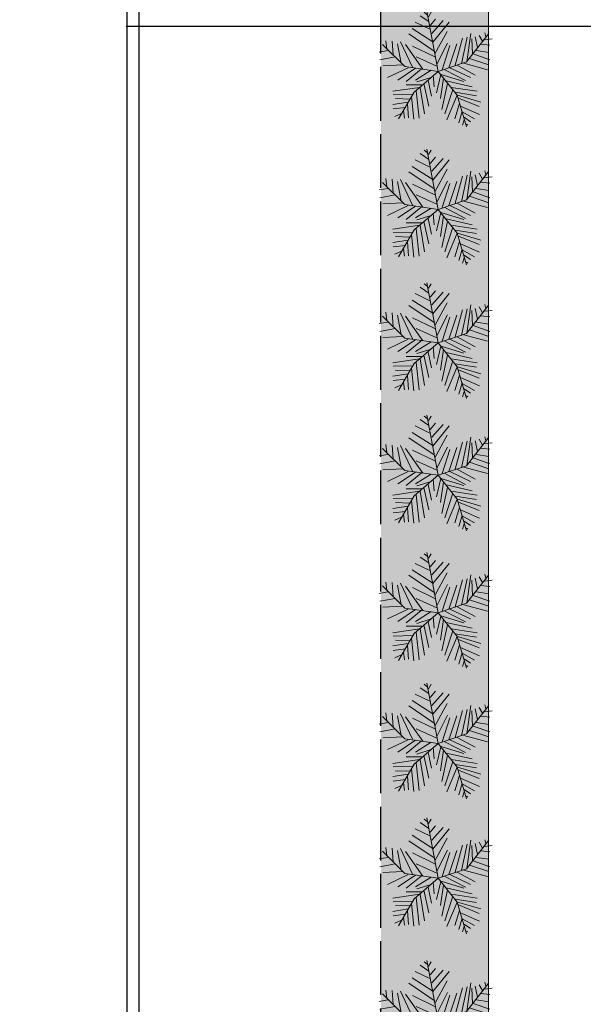
# Model space of a CAD drawing. Units: inches. Extents: x 853 to 1550, y 485 to 1596.
# Tile 12 of 18: x 853 to 979, y 1208 to 1428. Entities that reach past the tile are written whole.
import ezdxf

# ---------------------------------------------------------------- set-up
doc = ezdxf.new("R2010")
doc.units = ezdxf.units.IN
doc.header["$MEASUREMENT"] = 0
doc.linetypes.add('ACAD_ISO02W100', pattern=[15, 12, -3])
for name, color, linetype, lineweight in [('A-ANNO-DIMS', 2, 'Continuous', 18), ('C-PROP', 8, 'ACAD_ISO02W100', 25), ('L-PLNT-TREE', 106, 'Continuous', 13), ('lawn', 106, 'Continuous', 18)]:
    doc.layers.add(name, color=color, linetype=linetype, lineweight=lineweight)
doc.layers.add('L-PLNT-PATT', color=85, linetype='Continuous', lineweight=13, true_color=0x58ba48)
doc.styles.get("Standard").update_dxf_attribs({"font": 'arial.ttf'})
doc.dimstyles.get("Standard").update_dxf_attribs({"dimtxt": 8, "dimasz": 0.18, "dimexe": 0.18, "dimexo": 0.0625, "dimgap": 0.09, "dimtad": 0, "dimtih": 1, "dimtoh": 1, "dimzin": 0, "dimdsep": 46, "dimlunit": 3, "dimtxsty": 'Standard', "dimcen": 0.09, "dimadec": 0, "dimazin": 0, "dimtfac": 1, "dimtofl": 0, "dimtmove": 0, "dimatfit": 3, "dimfxl": 1, "dimtolj": 1, "dimtzin": 0, "dimarcsym": 0})

# ---------------------------------------------------------------- blocks, each defined once
blk = doc.blocks.new('*U18')
for p, q in [((-10.186, 53.64), (-13.084, 55.962)), ((0, 0), (-10.5, 57)), ((-9.099, 51.782), (-6.563, 55.962)), ((-7.288, 39.707), (-21.778, 46.673)), ((-8.737, 47.138), (-17.069, 52.711)), ((-7.65, 43.423), (-2.578, 49.46)), ((-5.839, 35.992), (4.667, 48.067)), ((-5.114, 27.632), (10.463, 46.673)), ((-5.114, 28.097), (-24.676, 40.636)), ((-2.941, 16.486), (8.652, 37.85)), ((-48.585, 21.131), (-49.309, 29.026)), ((-43.513, 28.561), (-42.427, 15.558)), ((-35.544, 28.097), (-24.314, 3.947)), ((-3.665, 19.273), (-27.574, 35.527)), ((16.259, 5.805), (23.142, 31.348)), ((22.055, 7.198), (27.489, 32.277)), ((27, 9), (48, 36)), ((27.127, 9.056), (31.112, 35.992)), ((31.836, 30.883), (32.561, 16.486)), ((35.096, 32.741), (37.27, 22.524)), ((38.719, 34.134), (41.979, 28.561)), ((43.791, 29.954), (51.036, 30.883)), ((44.153, 36.456), (45.239, 32.741)), ((-47.498, 19.737), (-55.83, 18.344)), ((-31.5, 4.5), (-52.5, 25.5)), ((-38.442, 26.239), (-34.819, 7.663)), ((-14.533, 2.09), (-30.834, 25.31)), ((-24.314, 23.917), (-2.941, 13.7)), ((-1.129, 6.734), (9.014, 26.704)), ((3.942, 1.625), (11.187, 24.381)), ((10.101, 3.483), (17.708, 26.239)), ((36.183, 19.737), (48.137, 17.88)), ((40.53, 25.775), (48.862, 24.846)), ((-40.615, 13.7), (-55.105, 10.913)), ((-20.691, 13.7), (-1.129, 4.876)), ((29.662, 12.307), (48.137, 6.269)), ((33.285, 16.486), (48.862, 10.913)), ((-33.37, 6.269), (-52.207, 5.34)), ((-28.299, 3.483), (-47.86, -5.805)), ((-21.416, 3.018), (-38.079, -8.128)), ((0, 0), (-31.5, 4.5)), ((-15.982, 2.09), (-30.11, -9.521)), ((0, 0), (-22.5, -19.5)), ((-6.563, 1.161), (-21.416, -8.128)), ((0, 0), (27, 9)), ((0, 0), (18, -22.5)), ((6.478, 1.625), (26.04, -8.592)), ((11.187, 3.483), (30.749, -5.805)), ((18.07, 5.805), (35.096, -3.483)), ((24.229, 7.663), (46.688, 1.625)), ((-6.563, -5.805), (-19.967, -9.985)), ((-9.461, -8.592), (-6.201, -23.453)), ((-4.752, -3.483), (-3.665, -14.629)), ((2.493, -3.019), (-1.491, -20.202)), ((1.769, -2.555), (24.229, -9.521)), ((5.029, -6.27), (2.131, -25.775)), ((7.565, -9.056), (32.198, -14.629)), ((-17.431, -15.094), (-42.789, -18.809)), ((-15.257, -12.772), (-30.11, -12.772)), ((-20.691, -18.345), (-17.793, -44.352)), ((-17.069, -15.094), (-12.721, -40.172)), ((-13.446, -11.378), (-8.737, -32.741)), ((9.014, -11.378), (3.58, -35.992)), ((14.085, -16.951), (6.478, -40.172)), ((12.274, -15.094), (36.907, -18.809)), ((-24.314, -21.596), (-42.427, -22.06)), ((-26.849, -26.24), (-40.253, -25.775)), ((-22.5, -19.5), (-37.5, -45)), ((-25.038, -23.918), (-22.865, -45.281)), ((18.07, -22.524), (8.289, -45.745)), ((16.259, -19.738), (36.183, -22.989)), ((18, -22.5), (27, -52.5)), ((18.433, -22.524), (40.53, -29.026)), ((19.157, -25.311), (38.719, -33.206)), ((-28.299, -29.026), (-42.789, -31.348)), ((-30.834, -34.135), (-42.427, -35.528)), ((-32.646, -36.921), (-31.921, -44.352)), ((-29.023, -30.884), (-27.936, -43.887)), ((20.244, -30.419), (15.897, -44.816)), ((21.331, -32.741), (39.081, -40.636)), ((-34.457, -39.708), (-40.978, -42.494)), ((22.78, -37.85), (19.519, -48.532)), ((22.78, -38.314), (34.372, -44.816)), ((24.591, -45.745), (23.142, -50.854)), ((24.591, -43.423), (30.749, -47.603)), ((26.764, -49.925), (28.213, -50.854))]:
    blk.add_line(p, q)
blk = doc.blocks.new('*D23')
at = {"layer": 'A-ANNO-DIMS', "color": 0, "lineweight": -2, "transparency": 16777216}
for p, q in [((879.97, 1474.13), (879.75, 1474.13)), ((879.93, 1473.95), (879.93, 1049.11)), ((879.93, 615.92), (879.93, 1040.76)), ((879.97, 615.74), (879.75, 615.74))]:
    blk.add_line(p, q, dxfattribs=at)
at = {"layer": 'A-ANNO-DIMS', "color": 0, "transparency": 16777216}
for points in [[(879.9, 1473.95), (879.96, 1473.95), (879.93, 1474.13)], [(879.9, 615.92), (879.96, 615.92), (879.93, 615.74)]]:
    blk.add_solid(points, dxfattribs=at)
at = {"layer": 'Defpoints', "color": 0, "transparency": 16777216}
for p in [(880.03, 1474.13), (879.93, 615.74), (880.03, 615.74)]:
    blk.add_point(p, dxfattribs=at)
at = {"layer": 'A-ANNO-DIMS', "color": 0, "transparency": 16777216, "insert": (879.93, 1044.94), "char_height": 8, "attachment_point": 5}
blk.add_mtext("\\A1;60'", dxfattribs=at)
blk = doc.blocks.new('*D70')
at = {"layer": 'A-ANNO-DIMS', "color": 0, "lineweight": -2, "transparency": 16777216}
for p, q in [((981.87, 1426.13), (877.09, 1426.13)), ((877.27, 1425.95), (877.27, 1067.22)), ((877.27, 700.05), (877.27, 1058.77)), ((1110.88, 699.87), (877.09, 699.87))]:
    blk.add_line(p, q, dxfattribs=at)
at = {"layer": 'A-ANNO-DIMS', "color": 0, "transparency": 16777216}
for points in [[(877.24, 1425.95), (877.3, 1425.95), (877.27, 1426.13)], [(877.24, 700.05), (877.3, 700.05), (877.27, 699.87)]]:
    blk.add_solid(points, dxfattribs=at)
at = {"layer": 'Defpoints', "color": 0, "transparency": 16777216}
for p in [(981.94, 1426.13), (877.27, 699.87), (1110.94, 699.87)]:
    blk.add_point(p, dxfattribs=at)
at = {"layer": 'A-ANNO-DIMS', "color": 0, "transparency": 16777216, "insert": (877.27, 1063), "char_height": 8, "attachment_point": 5}
blk.add_mtext('\\A1;60\'-6 1/2"', dxfattribs=at)
blk = doc.blocks.new('*D71')
at = {"layer": 'A-ANNO-DIMS', "color": 0, "lineweight": -2, "transparency": 16777216}
for p, q in [((933.87, 1474.13), (877.09, 1474.13)), ((877.27, 1473.95), (877.27, 1015.66)), ((877.27, 549.16), (877.27, 1007.45)), ((933.87, 548.98), (877.09, 548.98))]:
    blk.add_line(p, q, dxfattribs=at)
at = {"layer": 'A-ANNO-DIMS', "color": 0, "transparency": 16777216}
for points in [[(877.24, 1473.95), (877.3, 1473.95), (877.27, 1474.13)], [(877.24, 549.16), (877.3, 549.16), (877.27, 548.98)]]:
    blk.add_solid(points, dxfattribs=at)
at = {"layer": 'Defpoints', "color": 0, "transparency": 16777216}
for p in [(877.27, 1474.13), (933.94, 1474.13), (933.94, 548.98)]:
    blk.add_point(p, dxfattribs=at)
at = {"layer": 'A-ANNO-DIMS', "color": 0, "transparency": 16777216, "insert": (877.27, 1011.55), "char_height": 8, "attachment_point": 5}
blk.add_mtext('\\A1;77\'-1"', dxfattribs=at)

msp = doc.modelspace()

# ---------------------------------------------------------------- hatches: boundary and pattern name
at = {"layer": 'L-PLNT-PATT'}
h = msp.add_hatch(color=256, dxfattribs=at)
h.dxf.hatch_style = 1
h.paths.add_polyline_path([(1461.937, 1474.129), (933.937, 1474.129), (933.937, 730.129), (933.937, 622.891), (941.686, 622.891), (941.686, 604.895), (957.937, 604.895), (957.937, 1450.129), (1437.937, 1450.129), (1437.937, 604.895), (1454.646, 604.895), (1454.646, 622.891), (1461.937, 622.891), (1461.937, 734.988)])

# ---------------------------------------------------------------- linework, layer by layer
at = {"layer": 'C-PROP'}
msp.add_line((933.937, 730.129), (933.937, 1474.129), dxfattribs=at)
at = {"layer": 'lawn'}
msp.add_line((957.937, 765.455), (957.937, 1450.129), dxfattribs=at)

# ---------------------------------------------------------------- block references
at = {"layer": 'L-PLNT-TREE', "xscale": 0.2357951711934384, "yscale": 0.2357951711934384, "zscale": 0.2357951711934384}
for p in [(946.691, 1416.133), (946.691, 1385.37), (946.691, 1355.559), (946.691, 1326.04), (946.691, 1295.37), (946.691, 1266.227), (946.691, 1236.17), (946.691, 1204.359)]:
    msp.add_blockref('*U18', p, dxfattribs=at)

# ---------------------------------------------------------------- dimensions: what is measured, and where the dimension line sits
at = {"layer": 'A-ANNO-DIMS'}
for base, p1, p2, picture, middle in [((877.2718, 1474.1293), (933.9371, 548.9788), (933.9371, 1474.1293), '*D71', (877.2718, 1011.5541)), ((877.272, 699.868), (981.937, 1426.129), (1110.94, 699.868), '*D70', (877.272, 1062.999))]:
    dim = msp.add_linear_dim(base=base, p1=p1, p2=p2, angle=90, dimstyle='Standard', override={"dimdec": 1, "dimlfac": 1, "dimrnd": 0, "dimzin": 1, "dimdsep": 46, "dimlunit": 4, "dimfrac": 2}, dxfattribs=at)
    dim.commit()
    dim.dimension.update_dxf_attribs({"geometry": picture, "text_midpoint": middle})
dim = msp.add_linear_dim(base=(879.933, 615.743), p1=(880.035, 1474.129), p2=(880.035, 615.743), angle=90, text="60'", dimstyle='Standard', override={"dimclrd": 0, "dimclre": 0, "dimclrt": 0}, dxfattribs=at)
dim.commit()
dim.dimension.update_dxf_attribs({"geometry": '*D23', "text_midpoint": (879.933, 1044.936)})

doc.saveas('drawing.dxf')
